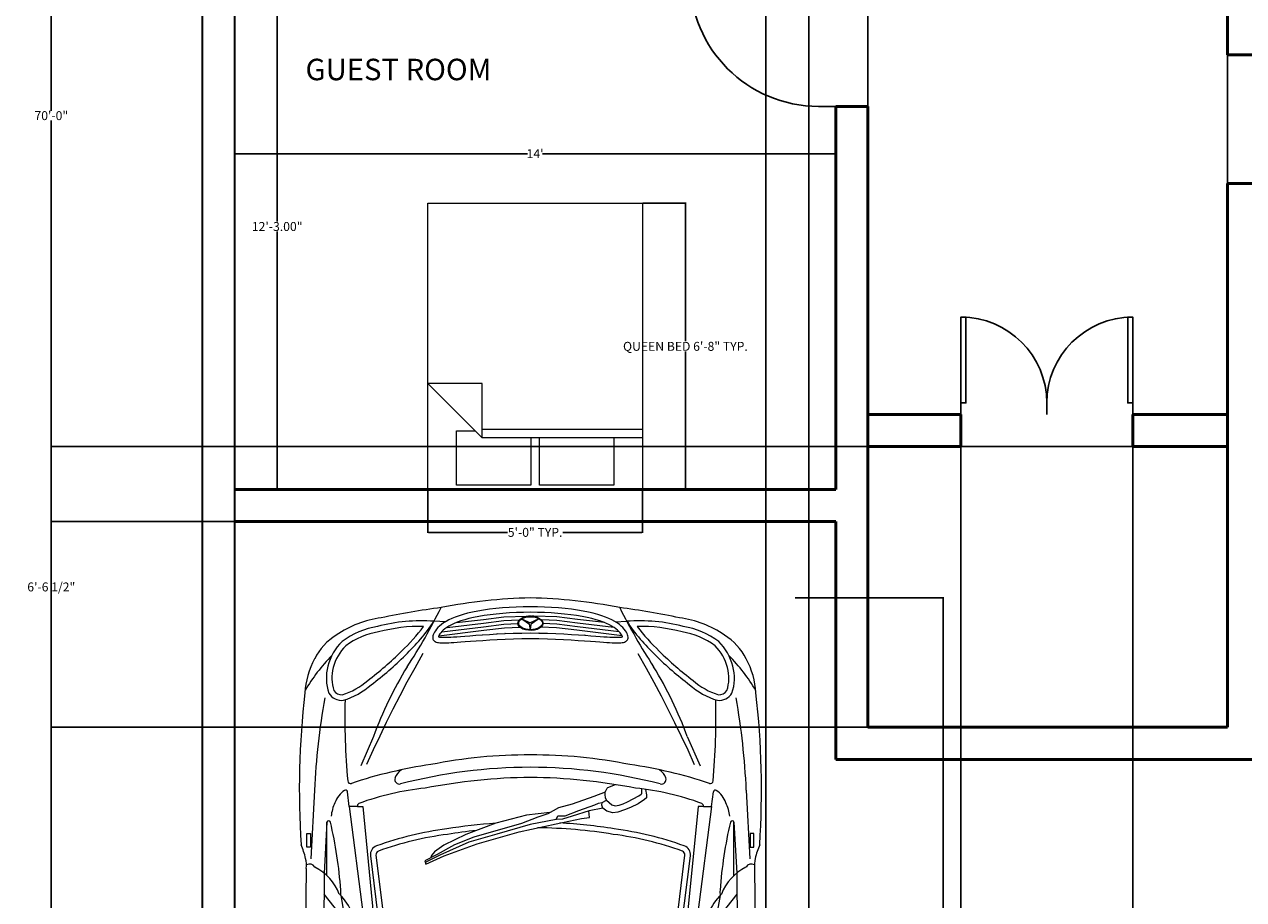
# Model space of a CAD drawing. Units: inches. Extents: x 594 to 1173, y 353 to 1285.
# Tile 2 of 6: x 594 to 934, y 600 to 844. Entities that reach past the tile are written whole.
import ezdxf

# ---------------------------------------------------------------- set-up
doc = ezdxf.new("R2010")
doc.units = ezdxf.units.IN
doc.header["$MEASUREMENT"] = 0
for name, color, linetype, lineweight in [('A-ANNO-DIMS', 2, 'Continuous', 18), ('A-AREA-IDEN', 7, 'Continuous', 25), ('A-DOOR', 4, 'Continuous', 25), ('A-FURN', 8, 'Continuous', 18), ('A-WALL', 7, 'Continuous', 50), ('C-PRKG-VEHI', 8, 'Continuous', 13), ('C-PROP', 7, 'Continuous', 35)]:
    doc.layers.add(name, color=color, linetype=linetype, lineweight=lineweight)
doc.styles.get("Standard").update_dxf_attribs({"font": 'arial.ttf'})
doc.dimstyles.get("Standard").update_dxf_attribs({"dimtxt": 2.5, "dimasz": 0.18, "dimexe": 0.18, "dimexo": 0.0625, "dimgap": 0.09, "dimtad": 0, "dimtih": 1, "dimtoh": 1, "dimzin": 0, "dimdsep": 46, "dimlunit": 3, "dimtxsty": 'Standard', "dimcen": 0.09, "dimadec": 0, "dimazin": 0, "dimtfac": 1, "dimtofl": 0, "dimtmove": 0, "dimatfit": 3, "dimfxl": 1, "dimtolj": 1, "dimtzin": 0, "dimarcsym": 0})

# ---------------------------------------------------------------- blocks, each defined once
blk = doc.blocks.new('*U2')
for p, q in [((0, 0), (0, -100)), ((750, 0), (750, -100))]:
    blk.add_line(p, q)
blk.add_lwpolyline([(0, 0), (0, 750), (43.75, 750), (43.75, 0)], close=True)
blk.add_arc((0, 0), 750, 0, 90)
blk = doc.blocks.new('Bed - Queen')
for p, q in [((0, -80.00003), (0, 0)), ((0, 0), (59.99999, 0)), ((59.99999, 0), (59.99999, -80.00003)), ((7.99999, -1.2), (28.79998, -1.2)), ((7.99999, -14.4), (7.99999, -1.2)), ((28.79998, -1.2), (28.79998, -14.4)), ((31.19999, -1.2), (51.99999, -1.2)), ((31.19999, -14.4), (31.19999, -1.2)), ((51.99999, -1.2), (51.99999, -16.4)), ((0, -14.4), (44.8, -14.4)), ((44.8, -16.8), (0, -16.8)), ((59.99999, -29.6), (44.8, -14.4)), ((44.8, -14.4), (44.8, -29.6)), ((51.99999, -16.4), (46.79936, -16.4)), ((44.8, -29.6), (59.99999, -29.6)), ((59.99999, -80.00003), (0, -80.00003))]:
    blk.add_line(p, q)
blk = doc.blocks.new('A$C27D64469')
for p, q in [((-0.0875, -0.4373), (-0.1114, -0.4395)), ((-0.0629, -0.4354), (-0.0875, -0.4373)), ((-0.0377, -0.4341), (-0.0629, -0.4354)), ((-0.0122, -0.4333), (-0.0377, -0.4341)), ((0.0136, -0.433), (-0.0122, -0.4333)), ((0.0393, -0.4333), (0.0136, -0.433)), ((0.0649, -0.4341), (0.0393, -0.4333)), ((0.0901, -0.4354), (0.0649, -0.4341)), ((0.1147, -0.4373), (0.0901, -0.4354)), ((0.1385, -0.4395), (0.1147, -0.4373)), ((-0.2803, -0.4806), (-0.2902, -0.486)), ((-0.2693, -0.4753), (-0.2803, -0.4806)), ((-0.2571, -0.4703), (-0.2693, -0.4753)), ((-0.2436, -0.4655), (-0.2571, -0.4703)), ((-0.253, -0.4902), (-0.1557, -0.4786)), ((-0.2289, -0.4609), (-0.2436, -0.4655)), ((-0.2233, -0.4801), (-0.2373, -0.4844)), ((-0.2128, -0.4566), (-0.2289, -0.4609)), ((-0.208, -0.476), (-0.2233, -0.4801)), ((-0.1954, -0.4525), (-0.2128, -0.4566)), ((-0.1912, -0.4721), (-0.208, -0.476)), ((-0.1764, -0.4487), (-0.1954, -0.4525)), ((-0.1728, -0.4684), (-0.1912, -0.4721)), ((-0.156, -0.4453), (-0.1764, -0.4487)), ((-0.153, -0.4651), (-0.1728, -0.4684)), ((-0.1343, -0.4422), (-0.156, -0.4453)), ((-0.1557, -0.4786), (-0.0819, -0.4693)), ((-0.1557, -0.4919), (-0.0819, -0.4825)), ((-0.1317, -0.4621), (-0.153, -0.4651)), ((-0.1114, -0.4395), (-0.1343, -0.4422)), ((-0.1093, -0.4594), (-0.1317, -0.4621)), ((-0.0858, -0.4572), (-0.1093, -0.4594)), ((-0.0616, -0.4554), (-0.0858, -0.4572)), ((-0.0819, -0.4693), (0.0012, -0.4665)), ((-0.0819, -0.4825), (-0.0265, -0.4807)), ((-0.0369, -0.4541), (-0.0616, -0.4554)), ((-0.0117, -0.4533), (-0.0369, -0.4541)), ((-0.0174, -0.4766), (0.0132, -0.4908)), ((-0.0174, -0.4766), (0.0101, -0.4961)), ((0.0136, -0.453), (-0.0117, -0.4533)), ((0.0012, -0.4665), (0.0067, -0.4665)), ((0.0445, -0.4762), (0.0132, -0.4908)), ((0.0389, -0.4533), (0.0136, -0.453)), ((0.0445, -0.4762), (0.0162, -0.4961)), ((0.0259, -0.4665), (0.0204, -0.4665)), ((0.109, -0.4693), (0.0259, -0.4665)), ((0.064, -0.4541), (0.0389, -0.4533)), ((0.109, -0.4825), (0.0537, -0.4807)), ((0.0888, -0.4554), (0.064, -0.4541)), ((0.113, -0.4572), (0.0888, -0.4554)), ((0.1828, -0.4786), (0.109, -0.4693)), ((0.1828, -0.4919), (0.109, -0.4825)), ((0.1364, -0.4594), (0.113, -0.4572)), ((0.1588, -0.4621), (0.1364, -0.4594)), ((0.1614, -0.4422), (0.1385, -0.4395)), ((0.1801, -0.4651), (0.1588, -0.4621)), ((0.1832, -0.4453), (0.1614, -0.4422)), ((0.2, -0.4684), (0.1801, -0.4651)), ((0.2801, -0.4902), (0.1828, -0.4786)), ((0.2036, -0.4487), (0.1832, -0.4453)), ((0.2183, -0.4721), (0.2, -0.4684)), ((0.2225, -0.4525), (0.2036, -0.4487)), ((0.2351, -0.476), (0.2183, -0.4721)), ((0.24, -0.4566), (0.2225, -0.4525)), ((0.2505, -0.4801), (0.2351, -0.476)), ((0.2561, -0.4609), (0.24, -0.4566)), ((0.2644, -0.4844), (0.2505, -0.4801)), ((0.2708, -0.4655), (0.2561, -0.4609)), ((0.2842, -0.4703), (0.2708, -0.4655)), ((0.2964, -0.4753), (0.2842, -0.4703)), ((0.3075, -0.4806), (0.2964, -0.4753)), ((0.3174, -0.486), (0.3075, -0.4806)), ((-0.3324, -0.5247), (-0.3351, -0.5296)), ((-0.2923, -0.4873), (-0.3337, -0.4857)), ((-0.329, -0.5195), (-0.3324, -0.5247)), ((-0.3248, -0.514), (-0.329, -0.5195)), ((-0.3198, -0.5085), (-0.3248, -0.514)), ((-0.3138, -0.5028), (-0.3198, -0.5085)), ((-0.3166, -0.5376), (-0.154, -0.5181)), ((-0.307, -0.4972), (-0.3138, -0.5028)), ((-0.3095, -0.5269), (-0.3127, -0.5311)), ((-0.3055, -0.5225), (-0.3095, -0.5269)), ((-0.2991, -0.4915), (-0.307, -0.4972)), ((-0.306, -0.5231), (-0.1557, -0.5051)), ((-0.3006, -0.5178), (-0.3055, -0.5225)), ((-0.2947, -0.513), (-0.3006, -0.5178)), ((-0.2902, -0.486), (-0.2991, -0.4915)), ((-0.288, -0.5082), (-0.2947, -0.513)), ((-0.2883, -0.5077), (-0.2883, -0.5077)), ((-0.2801, -0.5033), (-0.288, -0.5082)), ((-0.287, -0.5076), (-0.1557, -0.4919)), ((-0.2712, -0.4984), (-0.2801, -0.5033)), ((-0.2612, -0.4936), (-0.2712, -0.4984)), ((-0.2499, -0.489), (-0.2612, -0.4936)), ((-0.2373, -0.4844), (-0.2499, -0.489)), ((-0.1557, -0.5051), (-0.0819, -0.4958)), ((-0.154, -0.5181), (-0.0802, -0.5088)), ((-0.0819, -0.4958), (-0.0315, -0.4941)), ((-0.0802, -0.5088), (-0.0242, -0.5069)), ((0.0133, -0.5159), (0.0101, -0.4961)), ((0.0133, -0.5159), (0.0162, -0.4961)), ((0.1074, -0.5088), (0.0513, -0.5069)), ((0.109, -0.4958), (0.0586, -0.4941)), ((0.1811, -0.5181), (0.1074, -0.5088)), ((0.1828, -0.5051), (0.109, -0.4958)), ((0.3438, -0.5376), (0.1811, -0.5181)), ((0.3141, -0.5076), (0.1828, -0.4919)), ((0.3332, -0.5231), (0.1828, -0.5051)), ((0.277, -0.489), (0.2644, -0.4844)), ((0.2883, -0.4936), (0.277, -0.489)), ((0.2984, -0.4984), (0.2883, -0.4936)), ((0.3073, -0.5033), (0.2984, -0.4984)), ((0.3151, -0.5082), (0.3073, -0.5033)), ((0.3219, -0.513), (0.3151, -0.5082)), ((0.3262, -0.4915), (0.3174, -0.486)), ((0.3195, -0.4873), (0.3609, -0.4857)), ((0.3277, -0.5178), (0.3219, -0.513)), ((0.3341, -0.4972), (0.3262, -0.4915)), ((0.3326, -0.5225), (0.3277, -0.5178)), ((0.3367, -0.5269), (0.3326, -0.5225)), ((0.341, -0.5028), (0.3341, -0.4972)), ((0.3399, -0.5311), (0.3367, -0.5269)), ((0.3469, -0.5085), (0.341, -0.5028)), ((0.352, -0.514), (0.3469, -0.5085)), ((0.3562, -0.5195), (0.352, -0.514)), ((0.3596, -0.5247), (0.3562, -0.5195)), ((0.3622, -0.5296), (0.3596, -0.5247)), ((-0.3381, -0.5386), (-0.3386, -0.5425)), ((-0.3386, -0.5425), (-0.3385, -0.5462)), ((-0.3385, -0.5462), (-0.3378, -0.5495)), ((-0.3369, -0.5343), (-0.3381, -0.5386)), ((-0.3378, -0.5495), (-0.3364, -0.5524)), ((-0.3351, -0.5296), (-0.3369, -0.5343)), ((-0.3364, -0.5524), (-0.3345, -0.5549)), ((-0.3345, -0.5549), (-0.3321, -0.5571)), ((-0.3321, -0.5571), (-0.3292, -0.5589)), ((-0.3292, -0.5589), (-0.3258, -0.5604)), ((-0.3258, -0.5604), (-0.3219, -0.5615)), ((-0.3219, -0.5615), (-0.3175, -0.5623)), ((-0.318, -0.5407), (-0.3183, -0.5417)), ((-0.3183, -0.5417), (-0.3172, -0.542)), ((-0.3169, -0.5381), (-0.318, -0.5407)), ((-0.3175, -0.5623), (-0.3126, -0.5629)), ((-0.3172, -0.542), (-0.3144, -0.5426)), ((-0.3152, -0.5348), (-0.3169, -0.5381)), ((-0.3127, -0.5311), (-0.3152, -0.5348)), ((-0.3144, -0.5426), (-0.3108, -0.543)), ((-0.3126, -0.5629), (-0.3072, -0.5633)), ((-0.3108, -0.543), (-0.3063, -0.5433)), ((-0.3072, -0.5633), (-0.3014, -0.5634)), ((-0.3063, -0.5433), (-0.3012, -0.5434)), ((-0.3014, -0.5634), (-0.2951, -0.5634)), ((-0.3012, -0.5434), (-0.2953, -0.5434)), ((-0.2953, -0.5434), (-0.2888, -0.5433)), ((-0.2951, -0.5634), (-0.2882, -0.5633)), ((-0.2888, -0.5433), (-0.2815, -0.543)), ((-0.2882, -0.5633), (-0.2806, -0.563)), ((-0.2815, -0.543), (-0.2731, -0.5425)), ((-0.2806, -0.563), (-0.272, -0.5625)), ((-0.2731, -0.5425), (-0.2632, -0.5419)), ((-0.272, -0.5625), (-0.2619, -0.5619)), ((-0.2632, -0.5419), (-0.2517, -0.5411)), ((-0.2619, -0.5619), (-0.2503, -0.5611)), ((-0.2517, -0.5411), (-0.2382, -0.5402)), ((-0.2503, -0.5611), (-0.2367, -0.5601)), ((-0.2382, -0.5402), (-0.2225, -0.539)), ((-0.2367, -0.5601), (-0.221, -0.559)), ((-0.2225, -0.539), (-0.2042, -0.5376)), ((-0.221, -0.559), (-0.2027, -0.5576)), ((-0.2042, -0.5376), (-0.1833, -0.5361)), ((-0.2027, -0.5576), (-0.1818, -0.556)), ((-0.1832, -0.5361), (-0.1598, -0.5344)), ((-0.1818, -0.556), (-0.1584, -0.5544)), ((-0.1597, -0.5344), (-0.1342, -0.5327)), ((-0.1584, -0.5544), (-0.1329, -0.5527)), ((-0.1341, -0.5327), (-0.1069, -0.5311)), ((-0.1329, -0.5527), (-0.1057, -0.5511)), ((-0.1067, -0.5311), (-0.0781, -0.5297)), ((-0.1057, -0.5511), (-0.0771, -0.5496)), ((-0.0779, -0.5297), (-0.0482, -0.5285)), ((-0.0771, -0.5496), (-0.0475, -0.5485)), ((-0.048, -0.5285), (-0.0176, -0.5278)), ((-0.0475, -0.5485), (-0.0171, -0.5478)), ((-0.0173, -0.5278), (0.0134, -0.5275)), ((-0.0171, -0.5478), (0.0136, -0.5475)), ((0.0136, -0.5475), (0.0443, -0.5478)), ((0.0138, -0.5275), (0.0444, -0.5278)), ((0.0443, -0.5478), (0.0746, -0.5485)), ((0.0448, -0.5278), (0.0751, -0.5285)), ((0.0746, -0.5485), (0.1043, -0.5496)), ((0.0754, -0.5285), (0.105, -0.5297)), ((0.1043, -0.5496), (0.1329, -0.5511)), ((0.1052, -0.5297), (0.1339, -0.5311)), ((0.1329, -0.5511), (0.1601, -0.5527)), ((0.134, -0.5311), (0.1612, -0.5327)), ((0.1601, -0.5527), (0.1855, -0.5544)), ((0.1614, -0.5327), (0.1869, -0.5344)), ((0.1855, -0.5544), (0.2089, -0.556)), ((0.187, -0.5344), (0.2103, -0.5361)), ((0.2089, -0.556), (0.2299, -0.5576)), ((0.2104, -0.5361), (0.2314, -0.5376)), ((0.2299, -0.5576), (0.2481, -0.559)), ((0.2314, -0.5376), (0.2496, -0.539)), ((0.2481, -0.559), (0.2639, -0.5601)), ((0.2496, -0.539), (0.2653, -0.5402)), ((0.2639, -0.5601), (0.2775, -0.5611)), ((0.2653, -0.5402), (0.2788, -0.5411)), ((0.2775, -0.5611), (0.2891, -0.5619)), ((0.2788, -0.5411), (0.2904, -0.5419)), ((0.2891, -0.5619), (0.2991, -0.5625)), ((0.2904, -0.5419), (0.3002, -0.5425)), ((0.2991, -0.5625), (0.3078, -0.563)), ((0.3002, -0.5425), (0.3087, -0.543)), ((0.3078, -0.563), (0.3154, -0.5633)), ((0.3087, -0.543), (0.316, -0.5433)), ((0.3154, -0.5633), (0.3222, -0.5634)), ((0.316, -0.5433), (0.3225, -0.5434)), ((0.3222, -0.5634), (0.3285, -0.5634)), ((0.3225, -0.5434), (0.3283, -0.5434)), ((0.3283, -0.5434), (0.3335, -0.5433)), ((0.3285, -0.5634), (0.3344, -0.5633)), ((0.3335, -0.5433), (0.3379, -0.543)), ((0.3344, -0.5633), (0.3398, -0.5629)), ((0.3379, -0.543), (0.3416, -0.5426)), ((0.3398, -0.5629), (0.3446, -0.5623)), ((0.3423, -0.5348), (0.3399, -0.5311)), ((0.3416, -0.5426), (0.3444, -0.542)), ((0.3441, -0.5381), (0.3423, -0.5348)), ((0.3451, -0.5407), (0.3441, -0.5381)), ((0.3444, -0.542), (0.3454, -0.5417)), ((0.3446, -0.5623), (0.349, -0.5615)), ((0.3454, -0.5417), (0.3451, -0.5407)), ((0.349, -0.5615), (0.3529, -0.5604)), ((0.3529, -0.5604), (0.3563, -0.5589)), ((0.3563, -0.5589), (0.3593, -0.5571)), ((0.3593, -0.5571), (0.3617, -0.5549)), ((0.3617, -0.5549), (0.3636, -0.5524)), ((0.3641, -0.5343), (0.3622, -0.5296)), ((0.3636, -0.5524), (0.3649, -0.5495)), ((0.3653, -0.5386), (0.3641, -0.5343)), ((0.3649, -0.5495), (0.3656, -0.5462)), ((0.3658, -0.5425), (0.3653, -0.5386)), ((0.3656, -0.5462), (0.3658, -0.5425)), ((-0.3736, -0.602), (-0.4036, -0.6546)), ((0.4008, -0.602), (0.4307, -0.6546)), ((-0.4036, -0.6546), (-0.4313, -0.7051)), ((0.4307, -0.6546), (0.4585, -0.7051)), ((-0.4313, -0.7051), (-0.4574, -0.7542)), ((0.4585, -0.7051), (0.4846, -0.7542)), ((-0.4574, -0.7542), (-0.4822, -0.8025)), ((0.4846, -0.7542), (0.5094, -0.8025)), ((-0.4822, -0.8025), (-0.5062, -0.8507)), ((0.5094, -0.8025), (0.5333, -0.8507)), ((-0.5062, -0.8507), (-0.5297, -0.8995)), ((0.5333, -0.8507), (0.5568, -0.8995)), ((-0.552, -0.901), (-0.5982, -1.0071)), ((-0.5297, -0.8995), (-0.5532, -0.9495)), ((0.5568, -0.8995), (0.5804, -0.9495)), ((0.5791, -0.901), (0.6253, -1.0071)), ((-0.5532, -0.9495), (-0.5772, -1.0014)), ((0.5804, -0.9495), (0.6044, -1.0014)), ((-0.7646, -1.0944), (-0.7774, -1.3418)), ((0.2832, -1.1011), (0.2905, -1.0871)), ((0.2925, -1.0852), (0.3197, -1.0743)), ((0.4151, -1.1035), (0.4148, -1.0897)), ((0.4283, -1.0915), (0.4315, -1.1115)), ((0.7917, -1.0944), (0.8046, -1.3418)), ((-0.6398, -1.1535), (-0.646, -1.0999)), ((0.2417, -1.1168), (0.1646, -1.1448)), ((0.2832, -1.1011), (0.2417, -1.1168)), ((0.2457, -1.1477), (0.2589, -1.1408)), ((0.2589, -1.1408), (0.2722, -1.1385)), ((0.2711, -1.1491), (0.2722, -1.1385)), ((0.2722, -1.1385), (0.2873, -1.1305)), ((0.283, -1.1095), (0.2832, -1.1011)), ((0.2848, -1.1224), (0.283, -1.1095)), ((0.2873, -1.1305), (0.2848, -1.1224)), ((0.2873, -1.1305), (0.2969, -1.1395)), ((0.2969, -1.1395), (0.3069, -1.1474)), ((0.3475, -1.1443), (0.3634, -1.137)), ((0.3634, -1.137), (0.3841, -1.1257)), ((0.3841, -1.1257), (0.4048, -1.1143)), ((0.4254, -1.1287), (0.4022, -1.1436)), ((0.4048, -1.1143), (0.4131, -1.1088)), ((0.4131, -1.1088), (0.4151, -1.106)), ((0.4151, -1.106), (0.4151, -1.1035)), ((0.4315, -1.1216), (0.4254, -1.1287)), ((0.4315, -1.1115), (0.4315, -1.1216)), ((0.6669, -1.1535), (0.6731, -1.0999)), ((-0.6398, -1.1535), (-0.5904, -1.5351)), ((-0.61, -1.1535), (-0.6398, -1.1535)), ((-0.61, -1.1535), (-0.5908, -1.1535)), ((-0.5908, -1.1535), (-0.5454, -1.6151)), ((0, -1.1841), (-0.1108, -1.2136)), ((0.0839, -1.1753), (0, -1.1841)), ((0.0761, -1.1797), (0.0401, -1.1917)), ((0.1143, -1.158), (0.0761, -1.1797)), ((0.1069, -1.2008), (0.112, -1.1865)), ((0.112, -1.1865), (0.1383, -1.1871)), ((0.1646, -1.1448), (0.1143, -1.158)), ((0.1383, -1.1871), (0.188, -1.1683)), ((0.2252, -1.1688), (0.1635, -1.1877)), ((0.188, -1.1683), (0.2457, -1.1477)), ((0.2271, -1.1931), (0.2246, -1.169)), ((0.2744, -1.1592), (0.2252, -1.1688)), ((0.2744, -1.1592), (0.2711, -1.1491)), ((0.2895, -1.1703), (0.2744, -1.1592)), ((0.3107, -1.1759), (0.2895, -1.1703)), ((0.3069, -1.1474), (0.3193, -1.1504)), ((0.3289, -1.1738), (0.3107, -1.1759)), ((0.3193, -1.1504), (0.3339, -1.1491)), ((0.3526, -1.1658), (0.3289, -1.1738)), ((0.3339, -1.1491), (0.3475, -1.1443)), ((0.3745, -1.1567), (0.3526, -1.1658)), ((0.4022, -1.1436), (0.3745, -1.1567)), ((0.618, -1.1535), (0.5726, -1.6151)), ((0.6669, -1.1535), (0.6175, -1.5351)), ((0.6371, -1.1535), (0.618, -1.1535)), ((0.6371, -1.1535), (0.6669, -1.1535)), ((-0.7203, -1.2103), (-0.7302, -1.3933)), ((-0.7203, -1.4019), (-0.7203, -1.2103)), ((-0.1108, -1.2136), (-0.2189, -1.2538)), ((-0.0188, -1.2151), (-0.1903, -1.264)), ((0.013, -1.2184), (-0.1069, -1.2532)), ((-0.0266, -1.2451), (0.1062, -1.2154)), ((0.0401, -1.1917), (-0.0188, -1.2151)), ((0.1069, -1.2008), (0.013, -1.2184)), ((0.1062, -1.2154), (0.1972, -1.1964)), ((0.1298, -1.1986), (0.1069, -1.2008)), ((0.1635, -1.1877), (0.1298, -1.1986)), ((0.1972, -1.1964), (0.2271, -1.1931)), ((0.7474, -1.4019), (0.7474, -1.2103)), ((0.7474, -1.2103), (0.7573, -1.3933)), ((-0.7922, -1.2996), (-0.7922, -1.251)), ((-0.7922, -1.251), (-0.7785, -1.251)), ((-0.7785, -1.251), (-0.7785, -1.2996)), ((-0.2189, -1.2538), (-0.2983, -1.2922)), ((-0.1903, -1.264), (-0.2605, -1.2919)), ((-0.1069, -1.2532), (-0.2084, -1.2823)), ((-0.1789, -1.2879), (-0.0266, -1.2451)), ((0.8056, -1.251), (0.8056, -1.2996)), ((0.8193, -1.251), (0.8056, -1.251)), ((0.8193, -1.2996), (0.8193, -1.251)), ((-0.7785, -1.2996), (-0.7922, -1.2996)), ((-0.3323, -1.3172), (-0.343, -1.3297)), ((-0.2983, -1.2922), (-0.3323, -1.3172)), ((-0.2605, -1.2919), (-0.3222, -1.3262)), ((-0.2084, -1.2823), (-0.3128, -1.3287)), ((-0.2968, -1.3312), (-0.1789, -1.2879)), ((0.8056, -1.2996), (0.8193, -1.2996)), ((-0.563, -1.3311), (-0.5244, -1.6438)), ((-0.5431, -1.3287), (-0.5046, -1.6408)), ((-0.3222, -1.3262), (-0.3675, -1.3491)), ((-0.3675, -1.3491), (-0.363, -1.3611)), ((-0.3128, -1.3287), (-0.3653, -1.355)), ((-0.363, -1.3611), (-0.2968, -1.3312)), ((-0.343, -1.3297), (-0.345, -1.3377)), ((0.5317, -1.6408), (0.5703, -1.3287)), ((0.5515, -1.6438), (0.5901, -1.3311)), ((-0.7946, -1.3764), (-0.7975, -1.6481)), ((-0.7302, -1.3933), (-0.7314, -1.6155)), ((0.7573, -1.3933), (0.7586, -1.6155)), ((0.8217, -1.3764), (0.8246, -1.6481)), ((-0.7306, -1.4695), (-0.6539, -1.5666)), ((-0.6702, -1.4746), (-0.6539, -1.5666)), ((0.7578, -1.4695), (0.681, -1.5666)), ((0.6973, -1.4746), (0.681, -1.5666))]:
    blk.add_line(p, q)
for centre, radius, start, end in [((0.1265, -3.625), 3.2185, 97.7633, 101.6634), ((-2.1519, 0.4791), 2.0583, 326.7435, 333.6014), ((0.0637, -2.359), 1.9586, 91.468, 100.9476), ((-0.0366, -2.359), 1.9586, 79.0524, 88.532), ((-0.0994, -3.625), 3.2185, 78.3366, 82.2367), ((2.179, 0.4791), 2.0583, 206.3986, 213.2565), ((-0.471, -0.8549), 0.3855, 97.9189, 123.9683), ((0.4981, -0.8549), 0.3855, 56.0317, 82.0811), ((-0.4915, -0.79), 0.2893, 99.1695, 126.8677), ((-0.4915, -0.79), 0.2693, 98.9551, 126.5901), ((-0.3813, -1.088), 0.6042, 85.4848, 104.9936), ((-0.3813, -1.088), 0.5842, 89.0187, 105.0943), ((-0.9467, -0.0711), 0.72, 313.4908, 323.0478), ((-0.9467, -0.0711), 0.74, 313.509, 325.9238), ((0.4084, -1.088), 0.6042, 75.0064, 94.5152), ((0.9738, -0.0711), 0.74, 214.0762, 226.491), ((0.4084, -1.088), 0.5842, 74.9057, 90.9813), ((0.9738, -0.0711), 0.72, 216.9522, 226.5092), ((0.5186, -0.79), 0.2693, 53.4099, 81.0449), ((0.5186, -0.79), 0.2893, 53.1323, 80.8305), ((-0.5677, -0.7201), 0.2198, 122.6776, 153.2639), ((-0.5339, -0.6931), 0.1879, 134.257, 165.9979), ((-0.2027, -0.5576), 0.02, 94.2621, 94.2814), ((-0.1818, -0.556), 0.02, 94.094, 94.2621), ((-0.1584, -0.5544), 0.02, 93.7902, 94.094), ((-0.1329, -0.5527), 0.02, 93.3698, 93.7902), ((-0.1057, -0.5511), 0.02, 92.8387, 93.3698), ((-0.0771, -0.5496), 0.02, 92.1933, 92.8387), ((-0.0475, -0.5485), 0.02, 91.423, 92.1933), ((-0.0171, -0.5478), 0.02, 90.5101, 91.423), ((0.0136, -0.5475), 0.02, 89.4899, 90.5101), ((0.0443, -0.5478), 0.02, 88.577, 89.4899), ((0.0746, -0.5485), 0.02, 87.8067, 88.577), ((0.1043, -0.5496), 0.02, 87.1613, 87.8067), ((0.1329, -0.5511), 0.02, 86.6302, 87.1613), ((0.1601, -0.5527), 0.02, 86.2098, 86.6302), ((0.1855, -0.5544), 0.02, 85.906, 86.2098), ((0.2089, -0.556), 0.02, 85.7379, 85.906), ((0.2299, -0.5576), 0.02, 85.7186, 85.7379), ((0.5611, -0.6931), 0.1879, 14.0021, 45.743), ((0.5949, -0.7201), 0.2198, 26.7361, 57.3224), ((-0.2571, -1.0501), 0.6264, 135.2689, 149.8576), ((-0.5339, -0.6931), 0.1679, 134.6933, 166.0746), ((-1.2622, 0.2224), 1.1505, 306.8088, 314.8317), ((-1.2622, 0.2224), 1.1705, 306.853, 314.8203), ((1.2894, 0.2224), 1.1705, 225.1797, 233.147), ((1.2894, 0.2224), 1.1505, 225.1683, 233.1912), ((0.5611, -0.6931), 0.1679, 13.9254, 45.3067), ((0.2842, -1.0501), 0.6264, 30.1424, 44.7311), ((-0.5196, -0.7579), 0.2801, 150.7841, 177.1611), ((-0.5599, -0.6904), 0.1621, 164.7178, 199.3716), ((-0.5599, -0.6904), 0.1421, 164.6281, 198.5509), ((0.7633, -1.3808), 1.4001, 148.5187, 159.9579), ((-0.7362, -1.3808), 1.4001, 20.0421, 31.4813), ((0.587, -0.6904), 0.1421, 341.4491, 15.3719), ((0.587, -0.6904), 0.1621, 340.6284, 15.2822), ((0.5467, -0.7579), 0.2801, 2.8389, 29.2159), ((-0.7354, -0.5187), 0.2425, 286.9921, 312.0664), ((0.7625, -0.5187), 0.2425, 227.9336, 253.0079), ((2.2292, -1.0935), 3.0486, 173.4174, 183.7163), ((-0.6669, -0.7176), 0.053, 210.0698, 276.7845), ((-0.6669, -0.7176), 0.033, 213.0457, 274.1097), ((-0.7354, -0.5187), 0.2625, 286.5483, 311.8628), ((0.7625, -0.5187), 0.2625, 228.1372, 253.4517), ((0.694, -0.7176), 0.053, 263.2155, 329.9302), ((0.694, -0.7176), 0.033, 265.8903, 326.9543), ((-2.2021, -1.0935), 3.0486, 356.2837, 6.5826), ((1.7769, -1.2069), 2.544, 169.9235, 177.4667), ((1.7667, -0.8364), 2.422, 178.3888, 185.3284), ((-1.7396, -0.8364), 2.422, 354.6716, 1.6112), ((-1.7498, -1.2069), 2.544, 2.5333, 10.0765), ((-0.1068, -2.6471), 1.6622, 98.2339, 108.4059), ((0.0046, -2.7444), 1.777, 89.7096, 101.339), ((0.0226, -2.7444), 1.777, 78.661, 90.2904), ((0.1339, -2.6471), 1.6622, 71.5941, 81.7661), ((-0.4585, -1.0557), 0.0168, 161.7809, 284.512), ((-0.4223, -1.0677), 0.055, 122.1615, 161.7809), ((0.0163, -2.8903), 1.8782, 90.0843, 104.512), ((0.0393, -3.1787), 2.1304, 90.6925, 100.9626), ((0.0108, -2.8903), 1.8782, 75.488, 89.9157), ((-0.0122, -3.1787), 2.1304, 79.0374, 89.3075), ((0.4494, -1.0677), 0.055, 18.2191, 57.8385), ((0.4857, -1.0557), 0.0168, 255.488, 18.2191), ((-0.6033, -1.1719), 0.0933, 124.7249, 159.8848), ((-0.6527, -1.1007), 0.00673, 6.5512, 124.7249), ((-0.6348, -1.0604), 0.0101, 185.3284, 288.4059), ((-0.2611, -2.0848), 1.0031, 95.9948, 110.0315), ((0.294, -1.0889), 0.004, 111.8862, 152.6845), ((0.2882, -2.0848), 1.0031, 69.9685, 84.0052), ((0.6619, -1.0604), 0.0101, 251.5941, 354.6716), ((0.6798, -1.1007), 0.00673, 55.2751, 173.4488), ((0.6305, -1.1719), 0.0933, 20.1152, 55.2751), ((-0.5552, -1.2042), 0.1503, 154.6022, 174.0364), ((-0.5998, -1.1515), 0.0104, 118.0528, 191.1071), ((0.6269, -1.1515), 0.0104, 348.8929, 61.9472), ((0.5823, -1.2042), 0.1503, 5.9636, 25.3978), ((-0.7137, -1.2111), 0.00665, 15.5251, 172.9634), ((-2.218, -1.5637), 1.5518, 4.0302, 13.202), ((0.0017, -2.9892), 1.779, 93.6503, 99.3781), ((0.0254, -2.9892), 1.759, 80.6111, 89.5421), ((0.0254, -2.9892), 1.779, 80.6219, 86.9829), ((2.2452, -1.5637), 1.5518, 166.798, 175.9698), ((0.7408, -1.2111), 0.00665, 7.0366, 164.4749), ((-0.1308, -2.4351), 1.2114, 97.4669, 109.7935), ((-0.1308, -2.4351), 1.1914, 97.4508, 109.7935), ((0.0017, -2.9892), 1.759, 95.9707, 99.3889), ((0.1579, -2.4351), 1.1914, 70.2065, 82.5492), ((0.1579, -2.4351), 1.2114, 70.2065, 82.5331), ((-1.1013, -1.4136), 0.3132, 13.4845, 23.0084), ((-0.5296, -1.327), 0.0337, 109.7935, 187.0357), ((-0.5296, -1.327), 0.0137, 109.7935, 187.0357), ((0.5567, -1.327), 0.0137, 352.9643, 70.2065), ((0.5567, -1.327), 0.0337, 352.9643, 70.2065), ((1.1284, -1.4136), 0.3132, 156.9916, 166.5155), ((-0.8898, -1.3641), 0.096, 352.6385, 14.2173), ((-0.7831, -1.3832), 0.0225, 29.7837, 118.4161), ((0.8102, -1.3832), 0.0225, 61.5839, 150.2163), ((0.9169, -1.3641), 0.096, 165.7827, 187.3615), ((-0.8418, -1.5314), 0.1776, 20.2536, 63.8557), ((0.8689, -1.5314), 0.1776, 116.1443, 159.7464), ((-0.7826, -1.5905), 0.1615, 18.3646, 48.2784), ((-0.771, -1.4642), 0.1013, 354.1028, 5.3715), ((0.8098, -1.5905), 0.1615, 131.7216, 161.6354), ((0.7981, -1.4642), 0.1013, 174.6285, 185.8972)]:
    blk.add_arc(centre, radius, start, end)
blk.add_ellipse((0.014, -0.4925), major_axis=(-0.0426, 0), ratio=0.550187)
blk.add_open_spline([(-0.0315, -0.4925), (-0.0315, -0.5012), (-0.0242, -0.5089), (0.0098, -0.5237), (0.0496, -0.5174), (0.0659, -0.4821), (0.0357, -0.4635), (-0.0133, -0.4686), (-0.0315, -0.4789), (-0.0315, -0.4925)], degree=3, knots=[0, 0, 0, 0, 0.903923, 0.903923, 2.878844, 2.878844, 4.872977, 4.872977, 6.283185, 6.283185, 6.283185, 6.283185])
blk = doc.blocks.new('*D17')
at = {"layer": 'A-ANNO-DIMS', "color": 0, "lineweight": -2, "transparency": 16777216}
for p, q in [((652.4, 861.28), (664.44, 861.28)), ((664.26, 861.1), (664.26, 789.15)), ((664.26, 714.46), (664.26, 786.42)), ((652.4, 714.28), (664.44, 714.28))]:
    blk.add_line(p, q, dxfattribs=at)
at = {"layer": 'A-ANNO-DIMS', "color": 0, "transparency": 16777216}
for points in [[(664.23, 861.1), (664.29, 861.1), (664.26, 861.28)], [(664.23, 714.46), (664.29, 714.46), (664.26, 714.28)]]:
    blk.add_solid(points, dxfattribs=at)
at = {"layer": 'Defpoints', "color": 0, "transparency": 16777216}
for p in [(652.34, 861.28), (652.34, 714.28), (664.26, 714.28)]:
    blk.add_point(p, dxfattribs=at)
at = {"layer": 'A-ANNO-DIMS', "color": 0, "transparency": 16777216, "insert": (664.26, 787.78), "char_height": 2.5, "attachment_point": 5}
blk.add_mtext('\\A1;12\'-3.00"', dxfattribs=at)
blk = doc.blocks.new('*D18')
at = {"layer": 'A-ANNO-DIMS', "color": 0, "lineweight": -2, "transparency": 16777216}
for p, q in [((652.34, 714.35), (652.34, 808.32)), ((652.52, 808.14), (734.24, 808.14)), ((820.16, 808.14), (738.43, 808.14)), ((820.34, 714.35), (820.34, 808.32))]:
    blk.add_line(p, q, dxfattribs=at)
at = {"layer": 'A-ANNO-DIMS', "color": 0, "transparency": 16777216}
for points in [[(652.52, 808.17), (652.52, 808.11), (652.34, 808.14)], [(820.16, 808.17), (820.16, 808.11), (820.34, 808.14)]]:
    blk.add_solid(points, dxfattribs=at)
at = {"layer": 'Defpoints', "color": 0, "transparency": 16777216}
for p in [(820.34, 808.14), (652.34, 714.28), (820.34, 714.28)]:
    blk.add_point(p, dxfattribs=at)
at = {"layer": 'A-ANNO-DIMS', "color": 0, "transparency": 16777216, "insert": (736.34, 808.14), "char_height": 2.5, "attachment_point": 5}
blk.add_mtext("\\A1;14'", dxfattribs=at)
blk = doc.blocks.new('*D24')
at = {"layer": 'A-ANNO-DIMS', "color": 0, "lineweight": -2, "transparency": 16777216}
for p, q in [((766.4, 794.28), (778.52, 794.28)), ((778.34, 794.1), (778.34, 755.74)), ((778.34, 714.46), (778.34, 752.82)), ((766.4, 714.28), (778.52, 714.28))]:
    blk.add_line(p, q, dxfattribs=at)
at = {"layer": 'A-ANNO-DIMS', "color": 0, "transparency": 16777216}
for points in [[(778.31, 794.1), (778.37, 794.1), (778.34, 794.28)], [(778.31, 714.46), (778.37, 714.46), (778.34, 714.28)]]:
    blk.add_solid(points, dxfattribs=at)
at = {"layer": 'Defpoints', "color": 0, "transparency": 16777216}
for p in [(766.34, 794.28), (766.34, 714.28), (778.34, 714.28)]:
    blk.add_point(p, dxfattribs=at)
at = {"layer": 'A-ANNO-DIMS', "color": 0, "transparency": 16777216, "insert": (778.34, 754.28), "char_height": 2.5, "attachment_point": 5}
blk.add_mtext('\\A1;QUEEN BED 6\'-8" TYP.', dxfattribs=at)
blk = doc.blocks.new('*D25')
at = {"layer": 'A-ANNO-DIMS', "color": 0, "lineweight": -2, "transparency": 16777216}
for p, q in [((706.34, 714.22), (706.34, 702.1)), ((766.34, 714.22), (766.34, 702.1)), ((706.52, 702.28), (728.63, 702.28)), ((766.16, 702.28), (744.05, 702.28))]:
    blk.add_line(p, q, dxfattribs=at)
at = {"layer": 'A-ANNO-DIMS', "color": 0, "transparency": 16777216}
for points in [[(706.52, 702.31), (706.52, 702.25), (706.34, 702.28)], [(766.16, 702.31), (766.16, 702.25), (766.34, 702.28)]]:
    blk.add_solid(points, dxfattribs=at)
at = {"layer": 'Defpoints', "color": 0, "transparency": 16777216}
for p in [(706.34, 714.28), (766.34, 714.28), (706.34, 702.28)]:
    blk.add_point(p, dxfattribs=at)
at = {"layer": 'A-ANNO-DIMS', "color": 0, "transparency": 16777216, "insert": (736.34, 702.28), "char_height": 2.5, "attachment_point": 5}
blk.add_mtext('\\A1;5\'-0" TYP.', dxfattribs=at)
blk = doc.blocks.new('*D44')
at = {"layer": 'A-ANNO-DIMS', "color": 0, "lineweight": -2, "transparency": 16777216}
for p, q in [((808.99, 683.97), (850.58, 683.97)), ((850.4, 683.79), (850.4, 547.1)), ((850.4, 407.65), (850.4, 544.34)), ((808.99, 407.47), (850.58, 407.47))]:
    blk.add_line(p, q, dxfattribs=at)
at = {"layer": 'A-ANNO-DIMS', "color": 0, "transparency": 16777216}
for points in [[(850.37, 683.79), (850.43, 683.79), (850.4, 683.97)], [(850.37, 407.65), (850.43, 407.65), (850.4, 407.47)]]:
    blk.add_solid(points, dxfattribs=at)
at = {"layer": 'Defpoints', "color": 0, "transparency": 16777216}
for p in [(808.93, 683.97), (850.4, 683.97), (808.93, 407.47)]:
    blk.add_point(p, dxfattribs=at)
at = {"layer": 'A-ANNO-DIMS', "color": 0, "transparency": 16777216, "insert": (850.4, 545.72), "char_height": 2.5, "attachment_point": 5}
blk.add_mtext('\\A1;VEHICLE 23\'-0 1/2"', dxfattribs=at)
blk = doc.blocks.new('*D47')
at = {"layer": 'A-ANNO-DIMS', "color": 0, "lineweight": -2, "transparency": 16777216}
for p, q in [((643.27, 1238.78), (600.96, 1238.78)), ((601.14, 1238.6), (601.14, 820.15)), ((601.14, 398.96), (601.14, 817.42)), ((643.27, 398.78), (600.96, 398.78))]:
    blk.add_line(p, q, dxfattribs=at)
at = {"layer": 'A-ANNO-DIMS', "color": 0, "transparency": 16777216}
for points in [[(601.11, 1238.6), (601.17, 1238.6), (601.14, 1238.78)], [(601.11, 398.96), (601.17, 398.96), (601.14, 398.78)]]:
    blk.add_solid(points, dxfattribs=at)
at = {"layer": 'Defpoints', "color": 0, "transparency": 16777216}
for p in [(601.14, 1238.78), (643.34, 1238.78), (643.34, 398.78)]:
    blk.add_point(p, dxfattribs=at)
at = {"layer": 'A-ANNO-DIMS', "color": 0, "transparency": 16777216, "insert": (601.14, 818.78), "char_height": 2.5, "attachment_point": 5}
blk.add_mtext('\\A1;70\'-0"', dxfattribs=at)
blk = doc.blocks.new('*D56')
at = {"layer": 'A-ANNO-DIMS', "color": 0, "lineweight": -2, "transparency": 16777216}
for p, q in [((652.27, 705.28), (600.96, 705.28)), ((601.14, 705.1), (601.14, 557.92)), ((601.14, 407.96), (601.14, 555.15)), ((652.27, 407.78), (600.96, 407.78))]:
    blk.add_line(p, q, dxfattribs=at)
at = {"layer": 'A-ANNO-DIMS', "color": 0, "transparency": 16777216}
for points in [[(601.11, 705.1), (601.17, 705.1), (601.14, 705.28)], [(601.11, 407.96), (601.17, 407.96), (601.14, 407.78)]]:
    blk.add_solid(points, dxfattribs=at)
at = {"layer": 'Defpoints', "color": 0, "transparency": 16777216}
for p in [(601.14, 705.28), (652.34, 705.28), (652.34, 407.78)]:
    blk.add_point(p, dxfattribs=at)
at = {"layer": 'A-ANNO-DIMS', "color": 0, "transparency": 16777216, "insert": (601.14, 556.53), "char_height": 2.5, "attachment_point": 5}
blk.add_mtext('\\A1;24\'-9 1/2"', dxfattribs=at)
blk = doc.blocks.new('*D58')
at = {"layer": 'A-ANNO-DIMS', "color": 0, "lineweight": -2, "transparency": 16777216}
for p, q in [((829.34, 647.85), (829.34, 1281.16)), ((929.84, 647.85), (929.84, 1281.16)), ((829.52, 1280.98), (873.26, 1280.98)), ((929.66, 1280.98), (885.91, 1280.98))]:
    blk.add_line(p, q, dxfattribs=at)
at = {"layer": 'A-ANNO-DIMS', "color": 0, "transparency": 16777216}
for points in [[(829.52, 1281.01), (829.52, 1280.95), (829.34, 1280.98)], [(929.66, 1281.01), (929.66, 1280.95), (929.84, 1280.98)]]:
    blk.add_solid(points, dxfattribs=at)
at = {"layer": 'Defpoints', "color": 0, "transparency": 16777216}
for p in [(929.84, 1280.98), (829.34, 647.78), (929.84, 647.78)]:
    blk.add_point(p, dxfattribs=at)
at = {"layer": 'A-ANNO-DIMS', "color": 0, "transparency": 16777216, "insert": (879.59, 1280.98), "char_height": 2.5, "attachment_point": 5}
blk.add_mtext('\\A1;8\'-4 1/2"', dxfattribs=at)
blk = doc.blocks.new('*D59')
at = {"layer": 'A-ANNO-DIMS', "color": 0, "lineweight": -2, "transparency": 16777216}
for p, q in [((903.27, 726.26), (600.96, 726.26)), ((601.14, 726.08), (601.14, 688.4)), ((601.14, 647.96), (601.14, 685.64)), ((929.77, 647.78), (600.96, 647.78))]:
    blk.add_line(p, q, dxfattribs=at)
at = {"layer": 'A-ANNO-DIMS', "color": 0, "transparency": 16777216}
for points in [[(601.11, 726.08), (601.17, 726.08), (601.14, 726.26)], [(601.11, 647.96), (601.17, 647.96), (601.14, 647.78)]]:
    blk.add_solid(points, dxfattribs=at)
at = {"layer": 'Defpoints', "color": 0, "transparency": 16777216}
for p in [(601.14, 726.26), (903.34, 726.26), (929.84, 647.78)]:
    blk.add_point(p, dxfattribs=at)
at = {"layer": 'A-ANNO-DIMS', "color": 0, "transparency": 16777216, "insert": (601.14, 687.02), "char_height": 2.5, "attachment_point": 5}
blk.add_mtext('\\A1;6\'-6 1/2"', dxfattribs=at)
blk = doc.blocks.new('*D69')
at = {"layer": 'A-ANNO-DIMS', "color": 0, "lineweight": -2, "transparency": 16777216}
for p, q in [((855.34, 726.2), (855.34, 356.4)), ((903.34, 726.2), (903.34, 356.4)), ((855.52, 356.58), (875.87, 356.58)), ((903.16, 356.58), (882.8, 356.58))]:
    blk.add_line(p, q, dxfattribs=at)
at = {"layer": 'A-ANNO-DIMS', "color": 0, "transparency": 16777216}
for points in [[(855.52, 356.61), (855.52, 356.55), (855.34, 356.58)], [(903.16, 356.61), (903.16, 356.55), (903.34, 356.58)]]:
    blk.add_solid(points, dxfattribs=at)
at = {"layer": 'Defpoints', "color": 0, "transparency": 16777216}
for p in [(855.34, 726.26), (903.34, 726.26), (903.34, 356.58)]:
    blk.add_point(p, dxfattribs=at)
at = {"layer": 'A-ANNO-DIMS', "color": 0, "transparency": 16777216, "insert": (879.34, 356.58), "char_height": 2.5, "attachment_point": 5}
blk.add_mtext('\\A1;4\'-0"', dxfattribs=at)
blk = doc.blocks.new('*D73')
at = {"layer": 'A-ANNO-DIMS', "color": 0, "lineweight": -2, "transparency": 16777216}
for p, q in [((800.84, 870.22), (800.84, 356.4)), ((812.84, 870.22), (812.84, 356.4)), ((801.02, 356.58), (803.54, 356.58)), ((812.66, 356.58), (810.13, 356.58))]:
    blk.add_line(p, q, dxfattribs=at)
at = {"layer": 'A-ANNO-DIMS', "color": 0, "transparency": 16777216}
for points in [[(801.02, 356.61), (801.02, 356.55), (800.84, 356.58)], [(812.66, 356.61), (812.66, 356.55), (812.84, 356.58)]]:
    blk.add_solid(points, dxfattribs=at)
at = {"layer": 'Defpoints', "color": 0, "transparency": 16777216}
for p in [(800.84, 870.28), (812.84, 870.28), (812.84, 356.58)]:
    blk.add_point(p, dxfattribs=at)
at = {"layer": 'A-ANNO-DIMS', "color": 0, "transparency": 16777216, "insert": (806.84, 356.58), "char_height": 2.5, "attachment_point": 5}
blk.add_mtext('\\A1;1\'-0"', dxfattribs=at)

msp = doc.modelspace()

# ---------------------------------------------------------------- linework, layer by layer
at = {"layer": 'A-WALL'}
for p, q in [((929.837, 835.783), (929.837, 848.783)), ((938.837, 835.783), (929.837, 835.783)), ((820.337, 821.362), (820.337, 714.283)), ((829.337, 821.283), (820.337, 821.283)), ((829.337, 821.283), (829.337, 647.783)), ((929.837, 647.783), (929.837, 799.783)), ((929.837, 799.783), (938.837, 799.783)), ((829.337, 735.259), (855.337, 735.259)), ((855.337, 735.259), (855.337, 726.259)), ((903.337, 726.259), (903.337, 735.259)), ((903.337, 735.259), (929.837, 735.259)), ((829.337, 726.259), (855.337, 726.259)), ((903.337, 726.259), (929.837, 726.259)), ((820.337, 714.283), (652.337, 714.283)), ((820.337, 705.283), (652.337, 705.283)), ((820.337, 705.283), (820.337, 638.783)), ((829.337, 647.783), (929.837, 647.783)), ((820.337, 638.783), (1114.337, 638.783))]:
    msp.add_line(p, q, dxfattribs=at)
at = {"layer": 'C-PROP'}
for p, q in [((643.337, 1238.783), (643.337, 398.783)), ((652.337, 1229.783), (652.337, 407.783))]:
    msp.add_line(p, q, dxfattribs=at)

# ---------------------------------------------------------------- block references
at = {"layer": 'A-DOOR', "xscale": -0.0478936875771171, "yscale": 0.0478936875771171, "zscale": 0.0478936875771171, "rotation": 90}
msp.add_blockref('*U2', (815.547, 857.283), dxfattribs=at)
at = {"layer": 'A-DOOR', "yscale": 0.0319999999999999, "zscale": 0.0319999999999999}
for p, xscale in [((855.337, 738.459), 0.0319999999999999), ((903.337, 738.459), -0.0319999999999999)]:
    msp.add_blockref('*U2', p, dxfattribs=dict(at, xscale=xscale))
at = {"layer": 'A-FURN', "rotation": 180}
msp.add_blockref('Bed - Queen', (766.337, 714.283), dxfattribs=at)
at = {"layer": 'C-PRKG-VEHI', "xscale": 77.53069963048091, "yscale": 77.53069963048091, "zscale": 77.53069963048091}
msp.add_blockref('A$C27D64469', (733.975, 715.065), dxfattribs=at)

# ---------------------------------------------------------------- texts
at = {"layer": 'A-AREA-IDEN'}
msp.add_text('GUEST ROOM', height=6, dxfattribs=at).set_placement((672.169, 828.671))

# ---------------------------------------------------------------- dimensions: what is measured, and where the dimension line sits
at = {"layer": 'A-ANNO-DIMS'}
for base, p1, p2, override, picture, middle in [((929.837, 1280.983), (829.337, 647.783), (929.837, 647.783), {"dimdec": 1, "dimlfac": 1, "dimrnd": 0, "dimzin": 1, "dimdsep": 46, "dimlunit": 4, "dimfrac": 2}, '*D58', (879.587, 1280.983)), ((812.837, 356.583), (800.837, 870.283), (812.837, 870.283), {"dimdec": 1, "dimlfac": 1, "dimrnd": 0, "dimzin": 1, "dimdsep": 46, "dimlunit": 4, "dimfrac": 2}, '*D73', (806.837, 356.583)), ((820.337, 808.139), (652.337, 714.283), (820.337, 714.283), {"dimclrd": 0, "dimclre": 0, "dimclrt": 0}, '*D18', (736.337, 808.139)), ((903.337, 356.583), (855.337, 726.259), (903.337, 726.259), {"dimdec": 1, "dimlfac": 1, "dimrnd": 0, "dimzin": 1, "dimdsep": 46, "dimlunit": 4, "dimfrac": 2}, '*D69', (879.337, 356.583))]:
    dim = msp.add_linear_dim(base=base, p1=p1, p2=p2, dimstyle='Standard', override=override, dxfattribs=at)
    dim.commit()
    dim.dimension.update_dxf_attribs({"geometry": picture, "text_midpoint": middle})
for base, p1, p2, override, picture, middle in [((601.137, 1238.783), (643.337, 398.783), (643.337, 1238.783), {"dimdec": 1, "dimlfac": 1, "dimrnd": 0, "dimzin": 1, "dimdsep": 46, "dimlunit": 4, "dimfrac": 2}, '*D47', (601.137, 818.783)), ((664.26, 714.283), (652.337, 861.283), (652.337, 714.283), {"dimclrd": 0, "dimclre": 0, "dimclrt": 0}, '*D17', (664.26, 787.783)), ((601.137, 726.259), (929.837, 647.783), (903.337, 726.259), {"dimdec": 1, "dimlfac": 1, "dimrnd": 0, "dimzin": 1, "dimdsep": 46, "dimlunit": 4, "dimfrac": 2}, '*D59', (601.137, 687.021)), ((601.137, 705.283), (652.337, 407.783), (652.337, 705.283), {"dimdec": 1, "dimlfac": 1, "dimrnd": 0, "dimzin": 1, "dimdsep": 46, "dimlunit": 4, "dimfrac": 2}, '*D56', (601.137, 556.533))]:
    dim = msp.add_linear_dim(base=base, p1=p1, p2=p2, angle=90, dimstyle='Standard', override=override, dxfattribs=at)
    dim.commit()
    dim.dimension.update_dxf_attribs({"geometry": picture, "text_midpoint": middle})
for base, p1, p2, angle, text, picture, middle in [((778.337, 714.283), (766.337, 794.283), (766.337, 714.283), 270, 'QUEEN BED <> TYP.', '*D24', (778.337, 754.283)), ((706.337, 702.283), (766.337, 714.283), (706.337, 714.283), 180, '<> TYP.', '*D25', (736.337, 702.283)), ((850.401, 683.971), (808.926, 407.468), (808.926, 683.971), 90, 'VEHICLE <>', '*D44', (850.401, 545.719))]:
    dim = msp.add_linear_dim(base=base, p1=p1, p2=p2, angle=angle, text=text, dimstyle='Standard', override={"dimdec": 1, "dimlfac": 1, "dimrnd": 0, "dimzin": 1, "dimdsep": 46, "dimlunit": 4, "dimfrac": 2}, dxfattribs=at)
    dim.commit()
    dim.dimension.update_dxf_attribs({"geometry": picture, "text_midpoint": middle})

doc.saveas('drawing.dxf')
